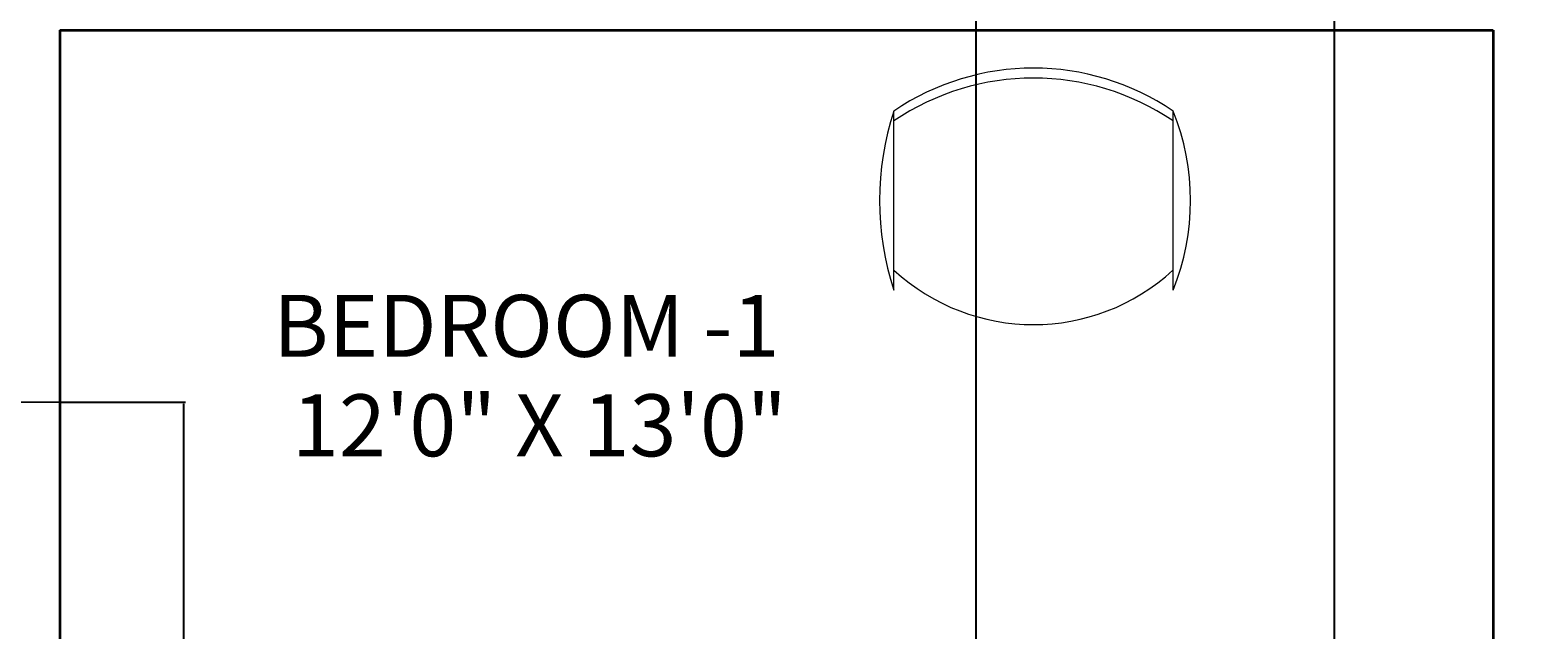
# Model space of a CAD drawing. Units: inches. Extents: x -61 to 1599, y -1316 to 257.
# Tile 123 of 204: x 85 to 236, y 88 to 149. Entities that reach past the tile are written whole.
import ezdxf

# ---------------------------------------------------------------- set-up
doc = ezdxf.new("R2010")
doc.units = ezdxf.units.IN
doc.header["$MEASUREMENT"] = 0
for name, color, linetype, lineweight in [('A-ANNO-DIMS', 2, 'Continuous', 18), ('A-AREA-IDEN', 1, 'Continuous', 18), ('FURNITURE', 83, 'Continuous', 18), ('WALLS', 4, 'Continuous', 35), ('WINDOWS', 220, 'Continuous', 18)]:
    doc.layers.add(name, color=color, linetype=linetype, lineweight=lineweight)
doc.styles.get("Standard").update_dxf_attribs({"font": 'arial.ttf'})
doc.dimstyles.get("Standard").update_dxf_attribs({"dimtxt": 0.18, "dimasz": 0.18, "dimexe": 0.18, "dimexo": 0.0625, "dimgap": 0.09, "dimtad": 0, "dimtih": 1, "dimtoh": 1, "dimdec": 0, "dimzin": 0, "dimdsep": 46, "dimlunit": 3, "dimtxsty": 'Standard', "dimcen": 0.09, "dimadec": 0, "dimazin": 0, "dimtfac": 1, "dimtdec": 0, "dimtofl": 0, "dimtmove": 0, "dimatfit": 3, "dimfxl": 1, "dimtolj": 1, "dimtzin": 0, "dimarcsym": 0})

# ---------------------------------------------------------------- blocks, each defined once
blk = doc.blocks.new('WIN-83IN')
for p, q in [((0, 82.94), (9, 82.94)), ((0, 0), (9, 0))]:
    blk.add_line(p, q)
for points in [[(9, 82.94), (4.5, 82.94), (4.5, 41.47), (9, 41.47)], [(4.5, 41.47), (0, 41.47), (0, 0), (4.5, 0)]]:
    blk.add_lwpolyline(points, close=True)
blk = doc.blocks.new('BEDROOM-CHAIR')
for p, q in [((1.45, 3.47), (1.45, 21.47)), ((29.49, 3.47), (29.49, 21.47))]:
    blk.add_line(p, q)
for centre, radius, start, end in [((15.47, 0.83), 24.95, 55.8098, 124.1902), ((15.47, -0.17), 24.95, 55.8098, 124.1902), ((28.58, 12.47), 28.58, 161.6455, 198.3545), ((7.26, 12.47), 23.99, 337.9646, 22.0354), ((15.47, 20.69), 20.68, 227.332, 312.668)]:
    blk.add_arc(centre, radius, start, end)
blk = doc.blocks.new('*D644')
at = {"layer": 'A-ANNO-DIMS', "color": 0, "lineweight": -2, "transparency": 16777216}
for p, q in [((87.77, 111.3), (100.32, 111.3)), ((100.14, 111.12), (100.14, 70.02)), ((100.14, 28.55), (100.14, 69.65)), ((87.77, 28.37), (100.32, 28.37))]:
    blk.add_line(p, q, dxfattribs=at)
at = {"layer": 'A-ANNO-DIMS', "color": 0, "transparency": 16777216}
for points in [[(100.11, 111.12), (100.17, 111.12), (100.14, 111.3)], [(100.11, 28.55), (100.17, 28.55), (100.14, 28.37)]]:
    blk.add_solid(points, dxfattribs=at)
at = {"layer": 'DEFPOINTS', "color": 0, "transparency": 16777216}
for p in [(87.7, 111.3), (100.14, 111.3), (87.7, 28.37)]:
    blk.add_point(p, dxfattribs=at)
at = {"layer": 'A-ANNO-DIMS', "color": 0, "transparency": 16777216, "insert": (100.14, 69.83), "char_height": 0.18, "attachment_point": 5}
blk.add_mtext('\\A1;WINDOW 83 TYP.', dxfattribs=at)
blk = doc.blocks.new('*D687')
at = {"layer": 'A-ANNO-DIMS', "color": 0, "lineweight": -2, "transparency": 16777216}
for p, q in [((289.42, 181.68), (-61.08, 181.68)), ((-60.9, 181.5), (-60.9, -528.95)), ((-60.9, -1239.76), (-60.9, -529.32)), ((319.64, -1239.94), (-61.08, -1239.94))]:
    blk.add_line(p, q, dxfattribs=at)
at = {"layer": 'A-ANNO-DIMS', "color": 0, "transparency": 16777216}
for points in [[(-60.93, 181.5), (-60.87, 181.5), (-60.9, 181.68)], [(-60.93, -1239.76), (-60.87, -1239.76), (-60.9, -1239.94)]]:
    blk.add_solid(points, dxfattribs=at)
at = {"layer": 'DEFPOINTS', "color": 0, "transparency": 16777216}
for p in [(289.48, 181.68), (-60.9, -1239.94), (319.7, -1239.94)]:
    blk.add_point(p, dxfattribs=at)
at = {"layer": 'A-ANNO-DIMS', "color": 0, "transparency": 16777216, "insert": (-60.9, -529.13), "char_height": 0.18, "attachment_point": 5}
blk.add_mtext('\\A1;1421.6', dxfattribs=at)
blk = doc.blocks.new('*D700')
at = {"layer": 'A-ANNO-DIMS', "color": 0, "lineweight": -2, "transparency": 16777216}
for p, q in [((14.7, -616.88), (14.7, 257.46)), ((14.88, 257.28), (96.77, 257.28)), ((179.57, 257.28), (97.68, 257.28)), ((179.75, -616.88), (179.75, 257.46))]:
    blk.add_line(p, q, dxfattribs=at)
at = {"layer": 'A-ANNO-DIMS', "color": 0, "transparency": 16777216}
for points in [[(14.88, 257.31), (14.88, 257.25), (14.7, 257.28)], [(179.57, 257.31), (179.57, 257.25), (179.75, 257.28)]]:
    blk.add_solid(points, dxfattribs=at)
at = {"layer": 'DEFPOINTS', "color": 0, "transparency": 16777216}
for p in [(179.75, 257.28), (14.7, -616.94), (179.75, -616.94)]:
    blk.add_point(p, dxfattribs=at)
at = {"layer": 'A-ANNO-DIMS', "color": 0, "transparency": 16777216, "insert": (97.23, 257.28), "char_height": 0.18, "attachment_point": 5}
blk.add_mtext('\\A1;165.05', dxfattribs=at)
blk = doc.blocks.new('*D701')
at = {"layer": 'A-ANNO-DIMS', "color": 0, "lineweight": -2, "transparency": 16777216}
for p, q in [((215.75, -616.88), (215.75, 257.46)), ((215.93, 257.28), (233.92, 257.28)), ((252.7, 257.28), (234.71, 257.28)), ((252.88, -616.88), (252.88, 257.46))]:
    blk.add_line(p, q, dxfattribs=at)
at = {"layer": 'A-ANNO-DIMS', "color": 0, "transparency": 16777216}
for points in [[(215.93, 257.31), (215.93, 257.25), (215.75, 257.28)], [(252.7, 257.31), (252.7, 257.25), (252.88, 257.28)]]:
    blk.add_solid(points, dxfattribs=at)
at = {"layer": 'DEFPOINTS', "color": 0, "transparency": 16777216}
for p in [(252.88, 257.28), (215.75, -616.94), (252.88, -616.94)]:
    blk.add_point(p, dxfattribs=at)
at = {"layer": 'A-ANNO-DIMS', "color": 0, "transparency": 16777216, "insert": (234.32, 257.28), "char_height": 0.18, "attachment_point": 5}
blk.add_mtext('\\A1;37.13', dxfattribs=at)

msp = doc.modelspace()

# ---------------------------------------------------------------- linework, layer by layer
at = {"layer": 'WALLS'}
for p, q in [((87.7028, 148.6771), (87.7028, -7.3229)), ((87.7028, 148.6771), (231.7028, 148.6771)), ((231.7028, 148.6771), (231.7028, -7.3229))]:
    msp.add_line(p, q, dxfattribs=at)

# ---------------------------------------------------------------- block references
at = {"layer": 'FURNITURE'}
msp.add_blockref('BEDROOM-CHAIR', (170.039, 119.079), dxfattribs=at)
at = {"layer": 'WINDOWS'}
msp.add_blockref('WIN-83IN', (78.703, 28.365), dxfattribs=at)

# ---------------------------------------------------------------- texts
at = {"layer": 'A-AREA-IDEN'}
for s, height, p in [('BEDROOM -1', 6.22364, (109.1314, 115.8502)), (' 12\'0" X 13\'0"', 6.223643, (109.1314, 105.8525))]:
    msp.add_text(s, height=height, dxfattribs=at).set_placement(p)

# ---------------------------------------------------------------- dimensions: what is measured, and where the dimension line sits
at = {"layer": 'A-ANNO-DIMS'}
for base, p1, p2, picture, middle in [((179.7521, 257.2771), (14.7028, -616.9446), (179.7521, -616.9446), '*D700', (97.2274, 257.2771)), ((252.8825, 257.2771), (215.7521, -616.9446), (252.8825, -616.9446), '*D701', (234.3173, 257.2771))]:
    dim = msp.add_linear_dim(base=base, p1=p1, p2=p2, dimstyle='Standard', override={"dimdec": 2, "dimlfac": 1, "dimrnd": 0, "dimzin": 0, "dimdsep": 46, "dimlunit": 2}, dxfattribs=at)
    dim.commit()
    dim.dimension.update_dxf_attribs({"geometry": picture, "text_midpoint": middle})
dim = msp.add_linear_dim(base=(-60.8972, -1239.9446), p1=(289.4807, 181.6771), p2=(319.7028, -1239.9446), angle=90, dimstyle='Standard', override={"dimdec": 1, "dimlfac": 1, "dimrnd": 0, "dimzin": 0, "dimdsep": 46, "dimlunit": 2}, dxfattribs=at)
dim.commit()
dim.dimension.update_dxf_attribs({"geometry": '*D687', "text_midpoint": (-60.8972, -529.1337)})
dim = msp.add_linear_dim(base=(100.1432, 111.3013), p1=(87.7028, 28.3651), p2=(87.7028, 111.3013), angle=90, text='WINDOW <> TYP.', dimstyle='Standard', override={"dimdec": 0, "dimlfac": 1, "dimrnd": 0, "dimzin": 0, "dimdsep": 46, "dimlunit": 2}, dxfattribs=at)
dim.commit()
dim.dimension.update_dxf_attribs({"geometry": '*D644', "text_midpoint": (100.1432, 69.8332)})

doc.saveas('drawing.dxf')
